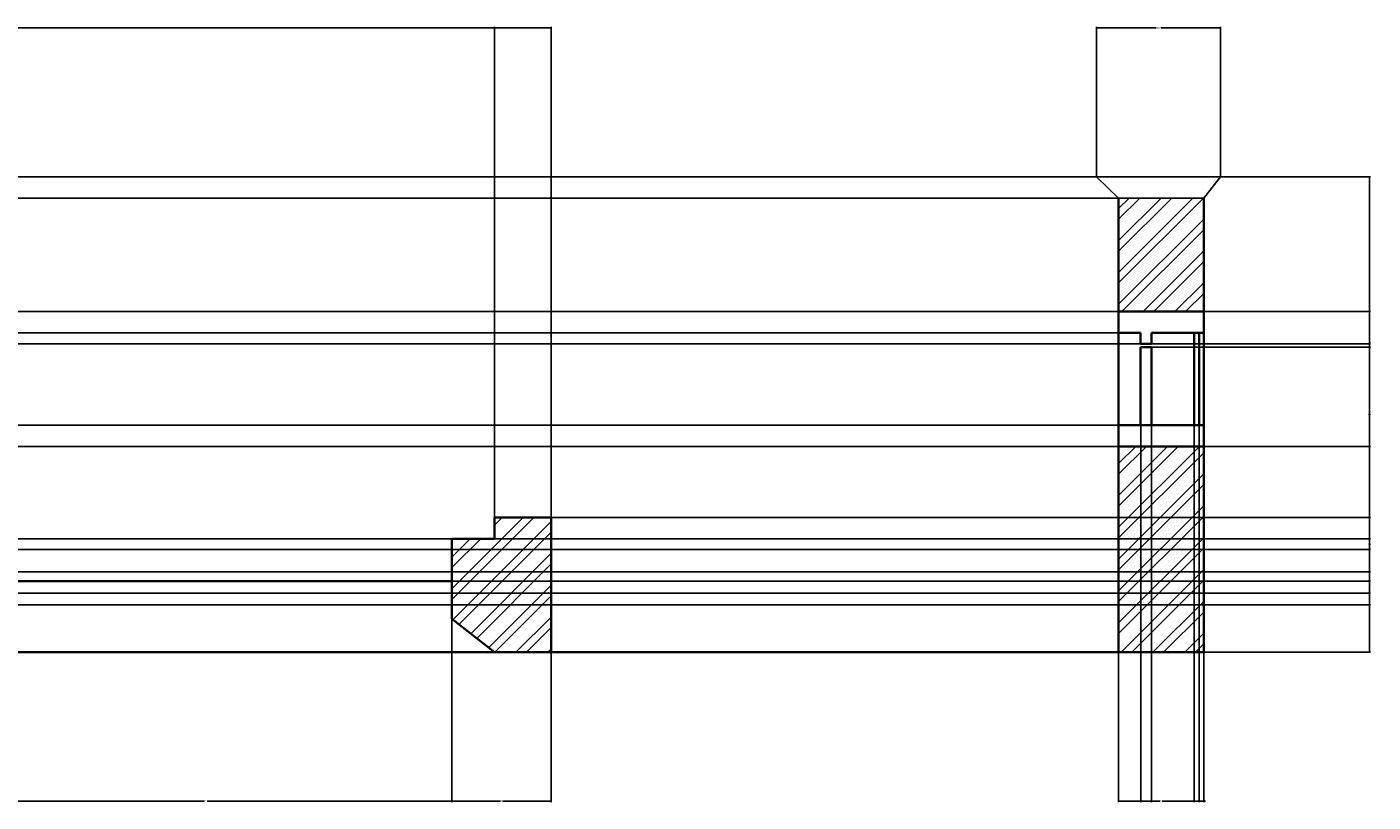
# Model space of a CAD drawing. Units: inches. Extents: x 2121 to 2815, y 1818 to 2233.
# Tile 6 of 6: x 2530 to 2815, y 2070 to 2233. Entities that reach past the tile are written whole.
import ezdxf

# ---------------------------------------------------------------- set-up
doc = ezdxf.new("R2010")
doc.units = ezdxf.units.IN
for name, color, linetype, lineweight in [('A-ANNO-DIMS', 2, 'Continuous', 18), ('A-COLS', 7, 'Continuous', 35), ('A-SECT', 7, 'Continuous', 35), ('A-WALL', 7, 'Continuous', 35), ('A-WALL-COPG', 7, 'Continuous', 25), ('A-WALL-PATT', 8, 'Continuous', 13)]:
    doc.layers.add(name, color=color, linetype=linetype, lineweight=lineweight)
doc.styles.get("Standard").update_dxf_attribs({"font": 'arial.ttf'})
doc.dimstyles.get("Standard").update_dxf_attribs({"dimtxt": 0.18, "dimasz": 0.18, "dimexe": 0.18, "dimexo": 0.0625, "dimgap": 0.09, "dimtad": 0, "dimtih": 1, "dimtoh": 1, "dimdec": 4, "dimzin": 0, "dimdsep": 46, "dimtxsty": 'Standard', "dimcen": 0.09, "dimadec": 0, "dimazin": 0, "dimtfac": 1, "dimtdec": 4, "dimtofl": 0, "dimtmove": 0, "dimatfit": 3, "dimfxl": 1, "dimtolj": 1, "dimtzin": 0, "dimarcsym": 0})

# ---------------------------------------------------------------- blocks, each defined once
blk = doc.blocks.new('*D10')
at = {"layer": 'A-ANNO-DIMS', "color": 0, "lineweight": -2, "transparency": 16777216}
for p, q in [((2152.83, 2129.87), (2152.83, 2233.48)), ((2153.01, 2233.3), (2396.54, 2233.3)), ((2640.65, 2233.3), (2397.13, 2233.3)), ((2640.83, 2129.87), (2640.83, 2233.48))]:
    blk.add_line(p, q, dxfattribs=at)
at = {"layer": 'A-ANNO-DIMS', "color": 0, "transparency": 16777216}
for points in [[(2153.01, 2233.33), (2153.01, 2233.27), (2152.83, 2233.3)], [(2640.65, 2233.33), (2640.65, 2233.27), (2640.83, 2233.3)]]:
    blk.add_solid(points, dxfattribs=at)
at = {"layer": 'Defpoints', "color": 0, "transparency": 16777216}
for p in [(2640.83, 2233.3), (2152.83, 2129.81), (2640.83, 2129.81)]:
    blk.add_point(p, dxfattribs=at)
at = {"layer": 'A-ANNO-DIMS', "color": 0, "transparency": 16777216, "insert": (2396.83, 2233.3), "char_height": 0.18, "attachment_point": 5}
blk.add_mtext('\\A1;488', dxfattribs=at)
blk = doc.blocks.new('*D11')
at = {"layer": 'A-ANNO-DIMS', "color": 0, "lineweight": -2, "transparency": 16777216}
for p, q in [((2640.9, 2129.81), (2814.07, 2129.81)), ((2813.89, 2129.63), (2813.89, 2115.74)), ((2813.89, 2101.49), (2813.89, 2115.38)), ((2640.9, 2101.31), (2814.07, 2101.31))]:
    blk.add_line(p, q, dxfattribs=at)
at = {"layer": 'A-ANNO-DIMS', "color": 0, "transparency": 16777216}
for points in [[(2813.86, 2129.63), (2813.92, 2129.63), (2813.89, 2129.81)], [(2813.86, 2101.49), (2813.92, 2101.49), (2813.89, 2101.31)]]:
    blk.add_solid(points, dxfattribs=at)
at = {"layer": 'Defpoints', "color": 0, "transparency": 16777216}
for p in [(2640.83, 2129.81), (2813.89, 2129.81), (2640.83, 2101.31)]:
    blk.add_point(p, dxfattribs=at)
at = {"layer": 'A-ANNO-DIMS', "color": 0, "transparency": 16777216, "insert": (2813.89, 2115.56), "char_height": 0.18, "attachment_point": 5}
blk.add_mtext('\\A1;28.5', dxfattribs=at)
blk = doc.blocks.new('*D26')
at = {"layer": 'A-ANNO-DIMS', "color": 0, "lineweight": -2, "transparency": 16777216}
for p, q in [((2515.83, 2116.25), (2515.83, 2069.63)), ((2619.83, 2108.3), (2619.83, 2069.63)), ((2516.01, 2069.81), (2567.55, 2069.81)), ((2619.65, 2069.81), (2568.11, 2069.81))]:
    blk.add_line(p, q, dxfattribs=at)
at = {"layer": 'A-ANNO-DIMS', "color": 0, "transparency": 16777216}
for points in [[(2516.01, 2069.84), (2516.01, 2069.78), (2515.83, 2069.81)], [(2619.65, 2069.84), (2619.65, 2069.78), (2619.83, 2069.81)]]:
    blk.add_solid(points, dxfattribs=at)
at = {"layer": 'Defpoints', "color": 0, "transparency": 16777216}
for p in [(2515.83, 2116.31), (2619.83, 2108.36), (2619.83, 2069.81)]:
    blk.add_point(p, dxfattribs=at)
at = {"layer": 'A-ANNO-DIMS', "color": 0, "transparency": 16777216, "insert": (2567.83, 2069.81), "char_height": 0.18, "attachment_point": 5}
blk.add_mtext('\\A1;104', dxfattribs=at)
blk = doc.blocks.new('*D27')
at = {"layer": 'A-ANNO-DIMS', "color": 0, "lineweight": -2, "transparency": 16777216}
for p, q in [((2619.83, 2108.3), (2619.83, 2069.63)), ((2640.83, 2101.25), (2640.83, 2069.63)), ((2620.01, 2069.81), (2630.13, 2069.81)), ((2640.65, 2069.81), (2630.54, 2069.81))]:
    blk.add_line(p, q, dxfattribs=at)
at = {"layer": 'A-ANNO-DIMS', "color": 0, "transparency": 16777216}
for points in [[(2620.01, 2069.84), (2620.01, 2069.78), (2619.83, 2069.81)], [(2640.65, 2069.84), (2640.65, 2069.78), (2640.83, 2069.81)]]:
    blk.add_solid(points, dxfattribs=at)
at = {"layer": 'Defpoints', "color": 0, "transparency": 16777216}
for p in [(2619.83, 2108.36), (2640.83, 2101.31), (2640.83, 2069.81)]:
    blk.add_point(p, dxfattribs=at)
at = {"layer": 'A-ANNO-DIMS', "color": 0, "transparency": 16777216, "insert": (2630.33, 2069.81), "char_height": 0.18, "attachment_point": 5}
blk.add_mtext('\\A1;21', dxfattribs=at)
blk = doc.blocks.new('*D32')
at = {"layer": 'A-ANNO-DIMS', "color": 0, "lineweight": -2, "transparency": 16777216}
for p, q in [((2311.9, 2113.81), (2814.07, 2113.81)), ((2813.89, 2113.63), (2813.89, 2112.74)), ((2813.89, 2111.49), (2813.89, 2112.38)), ((2311.9, 2111.31), (2814.07, 2111.31))]:
    blk.add_line(p, q, dxfattribs=at)
at = {"layer": 'A-ANNO-DIMS', "color": 0, "transparency": 16777216}
for points in [[(2813.86, 2113.63), (2813.92, 2113.63), (2813.89, 2113.81)], [(2813.86, 2111.49), (2813.92, 2111.49), (2813.89, 2111.31)]]:
    blk.add_solid(points, dxfattribs=at)
at = {"layer": 'Defpoints', "color": 0, "transparency": 16777216}
for p in [(2311.83, 2113.81), (2311.83, 2111.31), (2813.89, 2111.31)]:
    blk.add_point(p, dxfattribs=at)
at = {"layer": 'A-ANNO-DIMS', "color": 0, "transparency": 16777216, "insert": (2813.89, 2112.56), "char_height": 0.18, "attachment_point": 5}
blk.add_mtext('\\A1;2.5', dxfattribs=at)
blk = doc.blocks.new('*D33')
at = {"layer": 'A-ANNO-DIMS', "color": 0, "lineweight": -2, "transparency": 16777216}
for p, q in [((2386.9, 2118.31), (2814.07, 2118.31)), ((2813.89, 2118.13), (2813.89, 2116.24)), ((2813.89, 2113.99), (2813.89, 2115.88)), ((2386.9, 2113.81), (2814.07, 2113.81))]:
    blk.add_line(p, q, dxfattribs=at)
at = {"layer": 'A-ANNO-DIMS', "color": 0, "transparency": 16777216}
for points in [[(2813.86, 2118.13), (2813.92, 2118.13), (2813.89, 2118.31)], [(2813.86, 2113.99), (2813.92, 2113.99), (2813.89, 2113.81)]]:
    blk.add_solid(points, dxfattribs=at)
at = {"layer": 'Defpoints', "color": 0, "transparency": 16777216}
for p in [(2386.83, 2118.31), (2386.83, 2113.81), (2813.89, 2113.81)]:
    blk.add_point(p, dxfattribs=at)
at = {"layer": 'A-ANNO-DIMS', "color": 0, "transparency": 16777216, "insert": (2813.89, 2116.06), "char_height": 0.18, "attachment_point": 5}
blk.add_mtext('\\A1;4.5', dxfattribs=at)
blk = doc.blocks.new('*D34')
at = {"layer": 'A-ANNO-DIMS', "color": 0, "lineweight": -2, "transparency": 16777216}
for p, q in [((2515.9, 2116.31), (2814.07, 2116.31)), ((2813.89, 2116.13), (2813.89, 2108.99)), ((2813.89, 2101.49), (2813.89, 2108.63)), ((2500.9, 2101.31), (2814.07, 2101.31))]:
    blk.add_line(p, q, dxfattribs=at)
at = {"layer": 'A-ANNO-DIMS', "color": 0, "transparency": 16777216}
for points in [[(2813.86, 2116.13), (2813.92, 2116.13), (2813.89, 2116.31)], [(2813.86, 2101.49), (2813.92, 2101.49), (2813.89, 2101.31)]]:
    blk.add_solid(points, dxfattribs=at)
at = {"layer": 'Defpoints', "color": 0, "transparency": 16777216}
for p in [(2515.83, 2116.31), (2500.83, 2101.31), (2813.89, 2101.31)]:
    blk.add_point(p, dxfattribs=at)
at = {"layer": 'A-ANNO-DIMS', "color": 0, "transparency": 16777216, "insert": (2813.89, 2108.81), "char_height": 0.18, "attachment_point": 5}
blk.add_mtext('\\A1;15', dxfattribs=at)
blk = doc.blocks.new('*D35')
at = {"layer": 'A-ANNO-DIMS', "color": 0, "lineweight": -2, "transparency": 16777216}
for p, q in [((2628.83, 2129.87), (2628.83, 2233.48)), ((2629.01, 2233.3), (2634.62, 2233.3)), ((2640.65, 2233.3), (2635.04, 2233.3)), ((2640.83, 2129.87), (2640.83, 2233.48))]:
    blk.add_line(p, q, dxfattribs=at)
at = {"layer": 'A-ANNO-DIMS', "color": 0, "transparency": 16777216}
for points in [[(2629.01, 2233.33), (2629.01, 2233.27), (2628.83, 2233.3)], [(2640.65, 2233.33), (2640.65, 2233.27), (2640.83, 2233.3)]]:
    blk.add_solid(points, dxfattribs=at)
at = {"layer": 'Defpoints', "color": 0, "transparency": 16777216}
for p in [(2640.83, 2233.3), (2628.83, 2129.81), (2640.83, 2129.81)]:
    blk.add_point(p, dxfattribs=at)
at = {"layer": 'A-ANNO-DIMS', "color": 0, "transparency": 16777216, "insert": (2634.83, 2233.3), "char_height": 0.18, "attachment_point": 5}
blk.add_mtext('\\A1;12', dxfattribs=at)
blk = doc.blocks.new('*D39')
at = {"layer": 'A-ANNO-DIMS', "color": 0, "lineweight": -2, "transparency": 16777216}
for p, q in [((2515.9, 2125.31), (2814.07, 2125.31)), ((2813.89, 2125.13), (2813.89, 2124.33)), ((2813.89, 2123.17), (2813.89, 2123.97)), ((2511.4, 2122.99), (2814.07, 2122.99))]:
    blk.add_line(p, q, dxfattribs=at)
at = {"layer": 'A-ANNO-DIMS', "color": 0, "transparency": 16777216}
for points in [[(2813.86, 2125.13), (2813.92, 2125.13), (2813.89, 2125.31)], [(2813.86, 2123.17), (2813.92, 2123.17), (2813.89, 2122.99)]]:
    blk.add_solid(points, dxfattribs=at)
at = {"layer": 'Defpoints', "color": 0, "transparency": 16777216}
for p in [(2515.83, 2125.31), (2813.89, 2125.31), (2511.33, 2122.99)]:
    blk.add_point(p, dxfattribs=at)
at = {"layer": 'A-ANNO-DIMS', "color": 0, "transparency": 16777216, "insert": (2813.89, 2124.15), "char_height": 0.18, "attachment_point": 5}
blk.add_mtext('\\A1;2.314', dxfattribs=at)
blk = doc.blocks.new('*D83')
at = {"layer": 'A-ANNO-DIMS', "color": 0, "lineweight": -2, "transparency": 16777216}
for p, q in [((2756.14, 2201.87), (2756.14, 2233.48)), ((2756.32, 2233.3), (2768.8, 2233.3)), ((2782.21, 2233.3), (2769.73, 2233.3)), ((2782.39, 2201.87), (2782.39, 2233.48))]:
    blk.add_line(p, q, dxfattribs=at)
at = {"layer": 'A-ANNO-DIMS', "color": 0, "transparency": 16777216}
for points in [[(2756.32, 2233.33), (2756.32, 2233.27), (2756.14, 2233.3)], [(2782.21, 2233.33), (2782.21, 2233.27), (2782.39, 2233.3)]]:
    blk.add_solid(points, dxfattribs=at)
at = {"layer": 'Defpoints', "color": 0, "transparency": 16777216}
for p in [(2782.39, 2233.3), (2756.14, 2201.81), (2782.39, 2201.81)]:
    blk.add_point(p, dxfattribs=at)
at = {"layer": 'A-ANNO-DIMS', "color": 0, "transparency": 16777216, "insert": (2769.26, 2233.3), "char_height": 0.18, "attachment_point": 5}
blk.add_mtext('\\A1;26.255', dxfattribs=at)
blk = doc.blocks.new('*D84')
at = {"layer": 'A-ANNO-DIMS', "color": 0, "lineweight": -2, "transparency": 16777216}
for p, q in [((2760.83, 2101.25), (2760.83, 2069.63)), ((2778.83, 2101.25), (2778.83, 2069.63)), ((2761.01, 2069.81), (2769.62, 2069.81)), ((2778.65, 2069.81), (2770.04, 2069.81))]:
    blk.add_line(p, q, dxfattribs=at)
at = {"layer": 'A-ANNO-DIMS', "color": 0, "transparency": 16777216}
for points in [[(2761.01, 2069.84), (2761.01, 2069.78), (2760.83, 2069.81)], [(2778.65, 2069.84), (2778.65, 2069.78), (2778.83, 2069.81)]]:
    blk.add_solid(points, dxfattribs=at)
at = {"layer": 'Defpoints', "color": 0, "transparency": 16777216}
for p in [(2760.83, 2101.31), (2778.83, 2101.31), (2778.83, 2069.81)]:
    blk.add_point(p, dxfattribs=at)
at = {"layer": 'A-ANNO-DIMS', "color": 0, "transparency": 16777216, "insert": (2769.83, 2069.81), "char_height": 0.18, "attachment_point": 5}
blk.add_mtext('\\A1;18', dxfattribs=at)
blk = doc.blocks.new('*D85')
at = {"layer": 'A-ANNO-DIMS', "color": 0, "lineweight": -2, "transparency": 16777216}
for p, q in [((2782.45, 2201.81), (2814.07, 2201.81)), ((2813.89, 2201.63), (2813.89, 2151.74)), ((2813.89, 2101.49), (2813.89, 2151.38)), ((2778.9, 2101.31), (2814.07, 2101.31))]:
    blk.add_line(p, q, dxfattribs=at)
at = {"layer": 'A-ANNO-DIMS', "color": 0, "transparency": 16777216}
for points in [[(2813.86, 2201.63), (2813.92, 2201.63), (2813.89, 2201.81)], [(2813.86, 2101.49), (2813.92, 2101.49), (2813.89, 2101.31)]]:
    blk.add_solid(points, dxfattribs=at)
at = {"layer": 'Defpoints', "color": 0, "transparency": 16777216}
for p in [(2782.39, 2201.81), (2813.89, 2201.81), (2778.83, 2101.31)]:
    blk.add_point(p, dxfattribs=at)
at = {"layer": 'A-ANNO-DIMS', "color": 0, "transparency": 16777216, "insert": (2813.89, 2151.56), "char_height": 0.18, "attachment_point": 5}
blk.add_mtext('\\A1;100.5', dxfattribs=at)
blk = doc.blocks.new('*D86')
at = {"layer": 'A-ANNO-DIMS', "color": 0, "lineweight": -2, "transparency": 16777216}
for p, q in [((2760.77, 2144.81), (2121.16, 2144.81)), ((2121.34, 2144.63), (2121.34, 2123.24)), ((2121.34, 2101.49), (2121.34, 2122.88)), ((2760.77, 2101.31), (2121.16, 2101.31))]:
    blk.add_line(p, q, dxfattribs=at)
at = {"layer": 'A-ANNO-DIMS', "color": 0, "transparency": 16777216}
for points in [[(2121.31, 2144.63), (2121.37, 2144.63), (2121.34, 2144.81)], [(2121.31, 2101.49), (2121.37, 2101.49), (2121.34, 2101.31)]]:
    blk.add_solid(points, dxfattribs=at)
at = {"layer": 'Defpoints', "color": 0, "transparency": 16777216}
for p in [(2121.34, 2144.81), (2760.83, 2144.81), (2760.83, 2101.31)]:
    blk.add_point(p, dxfattribs=at)
at = {"layer": 'A-ANNO-DIMS', "color": 0, "transparency": 16777216, "insert": (2121.34, 2123.06), "char_height": 0.18, "attachment_point": 5}
blk.add_mtext('\\A1;43.5', dxfattribs=at)
blk = doc.blocks.new('*D87')
at = {"layer": 'A-ANNO-DIMS', "color": 0, "lineweight": -2, "transparency": 16777216}
for p, q in [((2778.9, 2173.31), (2814.07, 2173.31)), ((2813.89, 2173.13), (2813.89, 2159.24)), ((2813.89, 2144.99), (2813.89, 2158.88)), ((2778.9, 2144.81), (2814.07, 2144.81))]:
    blk.add_line(p, q, dxfattribs=at)
at = {"layer": 'A-ANNO-DIMS', "color": 0, "transparency": 16777216}
for points in [[(2813.86, 2173.13), (2813.92, 2173.13), (2813.89, 2173.31)], [(2813.86, 2144.99), (2813.92, 2144.99), (2813.89, 2144.81)]]:
    blk.add_solid(points, dxfattribs=at)
at = {"layer": 'Defpoints', "color": 0, "transparency": 16777216}
for p in [(2778.83, 2173.31), (2813.89, 2173.31), (2778.83, 2144.81)]:
    blk.add_point(p, dxfattribs=at)
at = {"layer": 'A-ANNO-DIMS', "color": 0, "transparency": 16777216, "insert": (2813.89, 2159.06), "char_height": 0.18, "attachment_point": 5}
blk.add_mtext('\\A1;28.5', dxfattribs=at)
blk = doc.blocks.new('*D88')
at = {"layer": 'A-ANNO-DIMS', "color": 0, "lineweight": -2, "transparency": 16777216}
for p, q in [((2760.77, 2197.31), (2121.16, 2197.31)), ((2121.34, 2197.13), (2121.34, 2185.49)), ((2121.34, 2173.49), (2121.34, 2185.13)), ((2760.77, 2173.31), (2121.16, 2173.31))]:
    blk.add_line(p, q, dxfattribs=at)
at = {"layer": 'A-ANNO-DIMS', "color": 0, "transparency": 16777216}
for points in [[(2121.31, 2197.13), (2121.37, 2197.13), (2121.34, 2197.31)], [(2121.31, 2173.49), (2121.37, 2173.49), (2121.34, 2173.31)]]:
    blk.add_solid(points, dxfattribs=at)
at = {"layer": 'Defpoints', "color": 0, "transparency": 16777216}
for p in [(2121.34, 2197.31), (2760.83, 2197.31), (2760.83, 2173.31)]:
    blk.add_point(p, dxfattribs=at)
at = {"layer": 'A-ANNO-DIMS', "color": 0, "transparency": 16777216, "insert": (2121.34, 2185.31), "char_height": 0.18, "attachment_point": 5}
blk.add_mtext('\\A1;24', dxfattribs=at)
blk = doc.blocks.new('*D89')
at = {"layer": 'A-ANNO-DIMS', "color": 0, "lineweight": -2, "transparency": 16777216}
for p, q in [((2756.07, 2201.81), (2121.16, 2201.81)), ((2121.34, 2201.63), (2121.34, 2199.74)), ((2121.34, 2197.49), (2121.34, 2199.38)), ((2760.77, 2197.31), (2121.16, 2197.31))]:
    blk.add_line(p, q, dxfattribs=at)
at = {"layer": 'A-ANNO-DIMS', "color": 0, "transparency": 16777216}
for points in [[(2121.31, 2201.63), (2121.37, 2201.63), (2121.34, 2201.81)], [(2121.31, 2197.49), (2121.37, 2197.49), (2121.34, 2197.31)]]:
    blk.add_solid(points, dxfattribs=at)
at = {"layer": 'Defpoints', "color": 0, "transparency": 16777216}
for p in [(2121.34, 2201.81), (2756.14, 2201.81), (2760.83, 2197.31)]:
    blk.add_point(p, dxfattribs=at)
at = {"layer": 'A-ANNO-DIMS', "color": 0, "transparency": 16777216, "insert": (2121.34, 2199.56), "char_height": 0.18, "attachment_point": 5}
blk.add_mtext('\\A1;4.5', dxfattribs=at)
blk = doc.blocks.new('*D90')
at = {"layer": 'A-ANNO-DIMS', "color": 0, "lineweight": -2, "transparency": 16777216}
for p, q in [((2760.77, 2168.81), (2121.16, 2168.81)), ((2121.34, 2168.63), (2121.34, 2159.24)), ((2121.34, 2149.49), (2121.34, 2158.88)), ((2760.77, 2149.31), (2121.16, 2149.31))]:
    blk.add_line(p, q, dxfattribs=at)
at = {"layer": 'A-ANNO-DIMS', "color": 0, "transparency": 16777216}
for points in [[(2121.31, 2168.63), (2121.37, 2168.63), (2121.34, 2168.81)], [(2121.31, 2149.49), (2121.37, 2149.49), (2121.34, 2149.31)]]:
    blk.add_solid(points, dxfattribs=at)
at = {"layer": 'Defpoints', "color": 0, "transparency": 16777216}
for p in [(2121.34, 2168.81), (2760.83, 2168.81), (2760.83, 2149.31)]:
    blk.add_point(p, dxfattribs=at)
at = {"layer": 'A-ANNO-DIMS', "color": 0, "transparency": 16777216, "insert": (2121.34, 2159.06), "char_height": 0.18, "attachment_point": 5}
blk.add_mtext('\\A1;19.5', dxfattribs=at)
blk = doc.blocks.new('*D91')
at = {"layer": 'A-ANNO-DIMS', "color": 0, "lineweight": -2, "transparency": 16777216}
for p, q in [((2760.77, 2149.31), (2121.16, 2149.31)), ((2121.34, 2149.13), (2121.34, 2147.24)), ((2121.34, 2144.99), (2121.34, 2146.88)), ((2760.77, 2144.81), (2121.16, 2144.81))]:
    blk.add_line(p, q, dxfattribs=at)
at = {"layer": 'A-ANNO-DIMS', "color": 0, "transparency": 16777216}
for points in [[(2121.31, 2149.13), (2121.37, 2149.13), (2121.34, 2149.31)], [(2121.31, 2144.99), (2121.37, 2144.99), (2121.34, 2144.81)]]:
    blk.add_solid(points, dxfattribs=at)
at = {"layer": 'Defpoints', "color": 0, "transparency": 16777216}
for p in [(2121.34, 2149.31), (2760.83, 2149.31), (2760.83, 2144.81)]:
    blk.add_point(p, dxfattribs=at)
at = {"layer": 'A-ANNO-DIMS', "color": 0, "transparency": 16777216, "insert": (2121.34, 2147.06), "char_height": 0.18, "attachment_point": 5}
blk.add_mtext('\\A1;4.5', dxfattribs=at)
blk = doc.blocks.new('*D92')
at = {"layer": 'A-ANNO-DIMS', "color": 0, "lineweight": -2, "transparency": 16777216}
for p, q in [((2760.83, 2149.25), (2760.83, 2069.63)), ((2765.49, 2149.25), (2765.49, 2069.63)), ((2761.01, 2069.81), (2762.76, 2069.81)), ((2765.31, 2069.81), (2763.56, 2069.81))]:
    blk.add_line(p, q, dxfattribs=at)
at = {"layer": 'A-ANNO-DIMS', "color": 0, "transparency": 16777216}
for points in [[(2761.01, 2069.84), (2761.01, 2069.78), (2760.83, 2069.81)], [(2765.31, 2069.84), (2765.31, 2069.78), (2765.49, 2069.81)]]:
    blk.add_solid(points, dxfattribs=at)
at = {"layer": 'Defpoints', "color": 0, "transparency": 16777216}
for p in [(2760.83, 2149.31), (2765.49, 2149.31), (2765.49, 2069.81)]:
    blk.add_point(p, dxfattribs=at)
at = {"layer": 'A-ANNO-DIMS', "color": 0, "transparency": 16777216, "insert": (2763.16, 2069.81), "char_height": 0.18, "attachment_point": 5}
blk.add_mtext('\\A1;4.654', dxfattribs=at)
blk = doc.blocks.new('*D93')
at = {"layer": 'A-ANNO-DIMS', "color": 0, "lineweight": -2, "transparency": 16777216}
for p, q in [((2765.49, 2149.25), (2765.49, 2069.63)), ((2767.8, 2149.25), (2767.8, 2069.63)), ((2765.67, 2069.81), (2766.25, 2069.81)), ((2767.62, 2069.81), (2767.04, 2069.81))]:
    blk.add_line(p, q, dxfattribs=at)
at = {"layer": 'A-ANNO-DIMS', "color": 0, "transparency": 16777216}
for points in [[(2765.67, 2069.84), (2765.67, 2069.78), (2765.49, 2069.81)], [(2767.62, 2069.84), (2767.62, 2069.78), (2767.8, 2069.81)]]:
    blk.add_solid(points, dxfattribs=at)
at = {"layer": 'Defpoints', "color": 0, "transparency": 16777216}
for p in [(2765.49, 2149.31), (2767.8, 2149.31), (2767.8, 2069.81)]:
    blk.add_point(p, dxfattribs=at)
at = {"layer": 'A-ANNO-DIMS', "color": 0, "transparency": 16777216, "insert": (2766.64, 2069.81), "char_height": 0.18, "attachment_point": 5}
blk.add_mtext('\\A1;2.313', dxfattribs=at)
blk = doc.blocks.new('*D94')
at = {"layer": 'A-ANNO-DIMS', "color": 0, "lineweight": -2, "transparency": 16777216}
for p, q in [((2776.8, 2149.25), (2776.8, 2069.63)), ((2777.83, 2149.25), (2777.83, 2069.63)), ((2776.62, 2069.81), (2776.44, 2069.81)), ((2778.01, 2069.81), (2778.19, 2069.81))]:
    blk.add_line(p, q, dxfattribs=at)
at = {"layer": 'A-ANNO-DIMS', "color": 0, "transparency": 16777216}
for points in [[(2776.62, 2069.84), (2776.62, 2069.78), (2776.8, 2069.81)], [(2778.01, 2069.84), (2778.01, 2069.78), (2777.83, 2069.81)]]:
    blk.add_solid(points, dxfattribs=at)
at = {"layer": 'Defpoints', "color": 0, "transparency": 16777216}
for p in [(2776.8, 2149.31), (2777.83, 2149.31), (2777.83, 2069.81)]:
    blk.add_point(p, dxfattribs=at)
at = {"layer": 'A-ANNO-DIMS', "color": 0, "transparency": 16777216, "insert": (2777.32, 2069.81), "char_height": 0.18, "attachment_point": 5}
blk.add_mtext('\\A1;1.02', dxfattribs=at)
blk = doc.blocks.new('*D95')
at = {"layer": 'A-ANNO-DIMS', "color": 0, "lineweight": -2, "transparency": 16777216}
for p, q in [((2777.827407, 2149.246525), (2777.827407, 2069.634025)), ((2778.832641, 2149.246525), (2778.832641, 2069.634025)), ((2777.647407, 2069.814025), (2777.467407, 2069.814025)), ((2779.012641, 2069.814025), (2779.192641, 2069.814025))]:
    blk.add_line(p, q, dxfattribs=at)
at = {"layer": 'A-ANNO-DIMS', "color": 0, "transparency": 16777216}
for points in [[(2777.647407, 2069.844025), (2777.647407, 2069.784025), (2777.827407, 2069.814025)], [(2779.012641, 2069.844025), (2779.012641, 2069.784025), (2778.832641, 2069.814025)]]:
    blk.add_solid(points, dxfattribs=at)
at = {"layer": 'Defpoints', "color": 0, "transparency": 16777216}
for p in [(2777.827407, 2149.309025), (2778.832641, 2149.309025), (2778.832641, 2069.814025)]:
    blk.add_point(p, dxfattribs=at)
at = {"layer": 'A-ANNO-DIMS', "color": 0, "transparency": 16777216, "insert": (2778.330024, 2069.814025), "char_height": 0.18, "attachment_point": 5}
blk.add_mtext('\\A1;1.01', dxfattribs=at)
blk = doc.blocks.new('*D96')
at = {"layer": 'A-ANNO-DIMS', "color": 0, "lineweight": -2, "transparency": 16777216}
for p, q in [((2767.86, 2166.48), (2814.07, 2166.48)), ((2813.89, 2166.48), (2813.89, 2166.66)), ((2813.89, 2166.66), (2814.07, 2166.66)), ((2813.89, 2165.96), (2813.89, 2166.3)), ((2767.86, 2165.78), (2814.07, 2165.78))]:
    blk.add_line(p, q, dxfattribs=at)
at = {"layer": 'A-ANNO-DIMS', "color": 0, "transparency": 16777216}
for points in [[(2813.86, 2166.3), (2813.92, 2166.3), (2813.89, 2166.48)], [(2813.86, 2165.96), (2813.92, 2165.96), (2813.89, 2165.78)]]:
    blk.add_solid(points, dxfattribs=at)
at = {"layer": 'Defpoints', "color": 0, "transparency": 16777216}
for p in [(2767.8, 2166.48), (2813.89, 2166.48), (2767.8, 2165.78)]:
    blk.add_point(p, dxfattribs=at)
at = {"layer": 'A-ANNO-DIMS', "color": 0, "transparency": 16777216, "insert": (2814.39, 2166.66), "char_height": 0.18, "attachment_point": 5}
blk.add_mtext('\\A1;0.70', dxfattribs=at)
blk = doc.blocks.new('*D97')
at = {"layer": 'A-ANNO-DIMS', "color": 0, "lineweight": -2, "transparency": 16777216}
for p, q in [((2765.42, 2168.81), (2121.16, 2168.81)), ((2765.42, 2166.48), (2121.16, 2166.48)), ((2121.34, 2168.63), (2121.34, 2167.83)), ((2121.34, 2166.66), (2121.34, 2167.46))]:
    blk.add_line(p, q, dxfattribs=at)
at = {"layer": 'A-ANNO-DIMS', "color": 0, "transparency": 16777216}
for points in [[(2121.31, 2168.63), (2121.37, 2168.63), (2121.34, 2168.81)], [(2121.31, 2166.66), (2121.37, 2166.66), (2121.34, 2166.48)]]:
    blk.add_solid(points, dxfattribs=at)
at = {"layer": 'Defpoints', "color": 0, "transparency": 16777216}
for p in [(2121.34, 2168.81), (2765.49, 2168.81), (2765.49, 2166.48)]:
    blk.add_point(p, dxfattribs=at)
at = {"layer": 'A-ANNO-DIMS', "color": 0, "transparency": 16777216, "insert": (2121.34, 2167.64), "char_height": 0.18, "attachment_point": 5}
blk.add_mtext('\\A1;2.33', dxfattribs=at)

msp = doc.modelspace()

# ---------------------------------------------------------------- hatches: boundary and pattern name
at = {"layer": 'A-WALL-PATT'}
h = msp.add_hatch(dxfattribs=at)
h.set_pattern_fill('ANSI32', color=256, scale=0.5)
h.paths.add_polyline_path([(2778.8326, 2197.309), (2760.8326, 2197.309), (2760.8326, 2173.309), (2778.8326, 2173.309)])
h.paths.add_polyline_path([(2778.8326, 2144.809), (2760.8326, 2144.809), (2760.8326, 2101.309), (2778.8326, 2101.309)])
h = msp.add_hatch(dxfattribs=at)
h.set_pattern_fill('ANSI32', color=256, scale=0.5)
h.paths.add_polyline_path([(2496.3326, 2122.9949), (2511.3326, 2122.9949), (2511.3326, 2117.8278), (2515.8326, 2122.3278), (2515.8326, 2125.309), (2157.3326, 2125.309), (2157.3326, 2129.809), (2152.8326, 2129.809), (2152.8326, 2125.309), (2152.8326, 2113.809), (2182.8326, 2113.809), (2182.8326, 2109.309), (2224.8326, 2109.309), (2224.8326, 2113.809), (2260.8326, 2113.809), (2260.8326, 2109.309), (2269.8326, 2109.309), (2269.8326, 2113.809), (2287.8326, 2113.809), (2287.8326, 2111.309), (2311.8326, 2111.309), (2311.8326, 2113.809), (2344.8326, 2113.809), (2344.8326, 2118.309), (2386.8326, 2118.309), (2386.8326, 2113.809), (2401.8326, 2113.809), (2401.8326, 2109.309), (2419.8326, 2109.309), (2419.8326, 2118.309), (2437.8326, 2118.309), (2437.8326, 2113.809), (2461.8326, 2113.809), (2461.8326, 2116.309), (2491.8326, 2116.309), (2491.8326, 2101.309), (2494.8138, 2101.309), (2496.3326, 2102.8278)])
h.paths.add_polyline_path([(2640.8326, 2129.809), (2628.8326, 2129.809), (2628.8326, 2125.309), (2619.8326, 2125.309), (2619.8326, 2108.3582), (2628.8326, 2101.309), (2640.8326, 2101.309)])

# ---------------------------------------------------------------- linework, layer by layer
at = {"layer": 'A-COLS'}
for p, q in [((2640.8326, 2129.809), (2628.8326, 2129.809)), ((2628.8326, 2129.809), (2628.8326, 2125.309)), ((2640.8326, 2101.309), (2640.8326, 2129.809)), ((2640.8326, 2125.309), (2640.8326, 2129.809)), ((2619.8326, 2108.3582), (2619.8326, 2125.309)), ((2619.8326, 2125.309), (2628.8326, 2125.309)), ((2628.8326, 2101.309), (2619.8326, 2108.3582)), ((2619.8326, 2101.309), (2628.8326, 2101.309))]:
    msp.add_line(p, q, dxfattribs=at)
at = {"layer": 'A-SECT'}
for p, q in [((2760.8326, 2101.309), (2760.8326, 2197.309)), ((2760.8326, 2173.309), (2760.8326, 2197.309)), ((2778.8326, 2101.309), (2778.8326, 2197.309)), ((2760.8326, 2149.309), (2760.8326, 2173.309)), ((2760.8326, 2173.309), (2778.8326, 2173.309)), ((2760.8326, 2168.809), (2765.4865, 2168.809)), ((2760.8326, 2168.809), (2765.4865, 2168.809)), ((2765.4865, 2168.809), (2765.4865, 2166.4788)), ((2765.4865, 2166.4788), (2767.7995, 2166.4788)), ((2767.7995, 2166.4788), (2767.7995, 2168.809)), ((2767.7995, 2168.809), (2778.8326, 2168.809)), ((2776.8035, 2149.309), (2776.8035, 2168.809)), ((2777.8274, 2168.809), (2777.8274, 2149.309)), ((2765.4865, 2165.7803), (2765.4865, 2149.309)), ((2765.4865, 2165.7803), (2767.7995, 2165.7803)), ((2767.7995, 2165.7803), (2767.7995, 2149.309)), ((2760.8326, 2101.309), (2760.8326, 2149.309)), ((2760.8326, 2149.309), (2778.8326, 2149.309)), ((2777.8274, 2149.309), (2776.8035, 2149.309)), ((2760.8326, 2144.809), (2778.8326, 2144.809))]:
    msp.add_line(p, q, dxfattribs=at)
at = {"layer": 'A-WALL'}
for p, q in [((2515.8326, 2116.309), (2619.8326, 2116.309)), ((2500.8326, 2101.309), (2778.8326, 2101.309))]:
    msp.add_line(p, q, dxfattribs=at)
at = {"layer": 'A-WALL-COPG'}
for p, q in [((2782.3922, 2201.809), (2756.1373, 2201.809)), ((2760.8326, 2197.309), (2756.1373, 2201.809)), ((2760.8326, 2201.809), (2778.8326, 2201.809)), ((2778.8326, 2197.309), (2782.3922, 2201.809)), ((2778.8326, 2201.809), (2782.3922, 2201.809)), ((2760.8326, 2197.309), (2778.8326, 2197.309))]:
    msp.add_line(p, q, dxfattribs=at)

# ---------------------------------------------------------------- dimensions: what is measured, and where the dimension line sits
at = {"layer": 'A-ANNO-DIMS'}
for base, p1, p2, override, picture, middle in [((2640.8326, 2233.304), (2152.8326, 2129.809), (2640.8326, 2129.809), {"dimdec": 0, "dimlfac": 1, "dimrnd": 0, "dimzin": 0, "dimdsep": 46, "dimlunit": 2}, '*D10', (2396.8326, 2233.304)), ((2640.8326, 2233.304), (2628.8326, 2129.809), (2640.8326, 2129.809), {"dimdec": 0, "dimlfac": 1, "dimrnd": 0, "dimzin": 0, "dimdsep": 46, "dimlunit": 2}, '*D35', (2634.8326, 2233.304)), ((2782.3922, 2233.304), (2756.1373, 2201.809), (2782.3922, 2201.809), {"dimdec": 3, "dimlfac": 1, "dimrnd": 0, "dimzin": 0, "dimdsep": 46, "dimlunit": 2}, '*D83', (2769.2648, 2233.304)), ((2765.4865, 2069.814), (2760.8326, 2149.309), (2765.4865, 2149.309), {"dimdec": 3, "dimlfac": 1, "dimrnd": 0, "dimzin": 0, "dimdsep": 46, "dimlunit": 2}, '*D92', (2763.1596, 2069.814)), ((2767.7995, 2069.814), (2765.4865, 2149.309), (2767.7995, 2149.309), {"dimdec": 3, "dimlfac": 1, "dimrnd": 0, "dimzin": 0, "dimdsep": 46, "dimlunit": 2}, '*D93', (2766.643, 2069.814)), ((2777.8274, 2069.814), (2776.8035, 2149.309), (2777.8274, 2149.309), {"dimdec": 2, "dimlfac": 1, "dimrnd": 0, "dimzin": 0, "dimdsep": 46, "dimlunit": 2}, '*D94', (2777.3155, 2069.814)), ((2778.8326, 2069.814), (2777.8274, 2149.309), (2778.8326, 2149.309), {"dimdec": 2, "dimlfac": 1, "dimrnd": 0, "dimzin": 0, "dimdsep": 46, "dimlunit": 2}, '*D95', (2778.33, 2069.814)), ((2619.8326, 2069.814), (2515.8326, 2116.309), (2619.8326, 2108.3582), {"dimdec": 0, "dimlfac": 1, "dimrnd": 0, "dimzin": 0, "dimdsep": 46, "dimlunit": 2}, '*D26', (2567.8326, 2069.814)), ((2640.8326, 2069.814), (2619.8326, 2108.3582), (2640.8326, 2101.309), {"dimdec": 0, "dimlfac": 1, "dimrnd": 0, "dimzin": 0, "dimdsep": 46, "dimlunit": 2}, '*D27', (2630.3326, 2069.814)), ((2778.8326, 2069.814), (2760.8326, 2101.309), (2778.8326, 2101.309), {"dimdec": 0, "dimlfac": 1, "dimrnd": 0, "dimzin": 0, "dimdsep": 46, "dimlunit": 2}, '*D84', (2769.8326, 2069.814))]:
    dim = msp.add_linear_dim(base=base, p1=p1, p2=p2, dimstyle='Standard', override=override, dxfattribs=at)
    dim.commit()
    dim.dimension.update_dxf_attribs({"geometry": picture, "text_midpoint": middle})
for base, p1, p2, override, picture, middle in [((2121.3376, 2201.809), (2760.8326, 2197.309), (2756.1373, 2201.809), {"dimdec": 1, "dimlfac": 1, "dimrnd": 0, "dimzin": 0, "dimdsep": 46, "dimlunit": 2}, '*D89', (2121.3376, 2199.559)), ((2813.8872, 2201.809), (2778.8326, 2101.309), (2782.3922, 2201.809), {"dimdec": 1, "dimlfac": 1, "dimrnd": 0, "dimzin": 0, "dimdsep": 46, "dimlunit": 2}, '*D85', (2813.8872, 2151.559)), ((2121.3376, 2197.309), (2760.8326, 2173.309), (2760.8326, 2197.309), {"dimdec": 0, "dimlfac": 1, "dimrnd": 0, "dimzin": 0, "dimdsep": 46, "dimlunit": 2}, '*D88', (2121.3376, 2185.309)), ((2813.8872, 2173.309), (2778.8326, 2144.809), (2778.8326, 2173.309), {"dimdec": 1, "dimlfac": 1, "dimrnd": 0, "dimzin": 0, "dimdsep": 46, "dimlunit": 2}, '*D87', (2813.8872, 2159.059)), ((2121.3376, 2168.809), (2760.8326, 2149.309), (2760.8326, 2168.809), {"dimdec": 1, "dimlfac": 1, "dimrnd": 0, "dimzin": 0, "dimdsep": 46, "dimlunit": 2}, '*D90', (2121.3376, 2159.059)), ((2121.3376, 2168.809), (2765.4865, 2166.4788), (2765.4865, 2168.809), {"dimdec": 2, "dimlfac": 1, "dimrnd": 0, "dimzin": 0, "dimdsep": 46, "dimlunit": 2}, '*D97', (2121.3376, 2167.6439)), ((2813.8872, 2166.4788), (2767.7995, 2165.7803), (2767.7995, 2166.4788), {"dimdec": 2, "dimlfac": 1, "dimrnd": 0, "dimzin": 0, "dimdsep": 46, "dimlunit": 2}, '*D96', (2814.3907, 2166.6588)), ((2121.3376, 2149.309), (2760.8326, 2144.809), (2760.8326, 2149.309), {"dimdec": 1, "dimlfac": 1, "dimrnd": 0, "dimzin": 0, "dimdsep": 46, "dimlunit": 2}, '*D91', (2121.3376, 2147.059)), ((2121.3376, 2144.809), (2760.8326, 2101.309), (2760.8326, 2144.809), {"dimdec": 1, "dimlfac": 1, "dimrnd": 0, "dimzin": 0, "dimdsep": 46, "dimlunit": 2}, '*D86', (2121.3376, 2123.059)), ((2813.8872, 2129.809), (2640.8326, 2101.309), (2640.8326, 2129.809), {"dimdec": 1, "dimlfac": 1, "dimrnd": 0, "dimzin": 0, "dimdsep": 46, "dimlunit": 2}, '*D11', (2813.8872, 2115.559)), ((2813.8872, 2125.309), (2511.3326, 2122.9949), (2515.8326, 2125.309), {"dimdec": 3, "dimlfac": 1, "dimrnd": 0, "dimzin": 0, "dimdsep": 46, "dimlunit": 2}, '*D39', (2813.8872, 2124.1519)), ((2813.8872, 2113.809), (2386.8326, 2118.309), (2386.8326, 2113.809), {"dimdec": 1, "dimlfac": 1, "dimrnd": 0, "dimzin": 0, "dimdsep": 46, "dimlunit": 2}, '*D33', (2813.8872, 2116.059)), ((2813.8872, 2101.309), (2515.8326, 2116.309), (2500.8326, 2101.309), {"dimdec": 0, "dimlfac": 1, "dimrnd": 0, "dimzin": 0, "dimdsep": 46, "dimlunit": 2}, '*D34', (2813.8872, 2108.809)), ((2813.8872, 2111.309), (2311.8326, 2113.809), (2311.8326, 2111.309), {"dimdec": 1, "dimlfac": 1, "dimrnd": 0, "dimzin": 0, "dimdsep": 46, "dimlunit": 2}, '*D32', (2813.8872, 2112.559))]:
    dim = msp.add_linear_dim(base=base, p1=p1, p2=p2, angle=90, dimstyle='Standard', override=override, dxfattribs=at)
    dim.commit()
    dim.dimension.update_dxf_attribs({"geometry": picture, "text_midpoint": middle})

doc.saveas('drawing.dxf')
